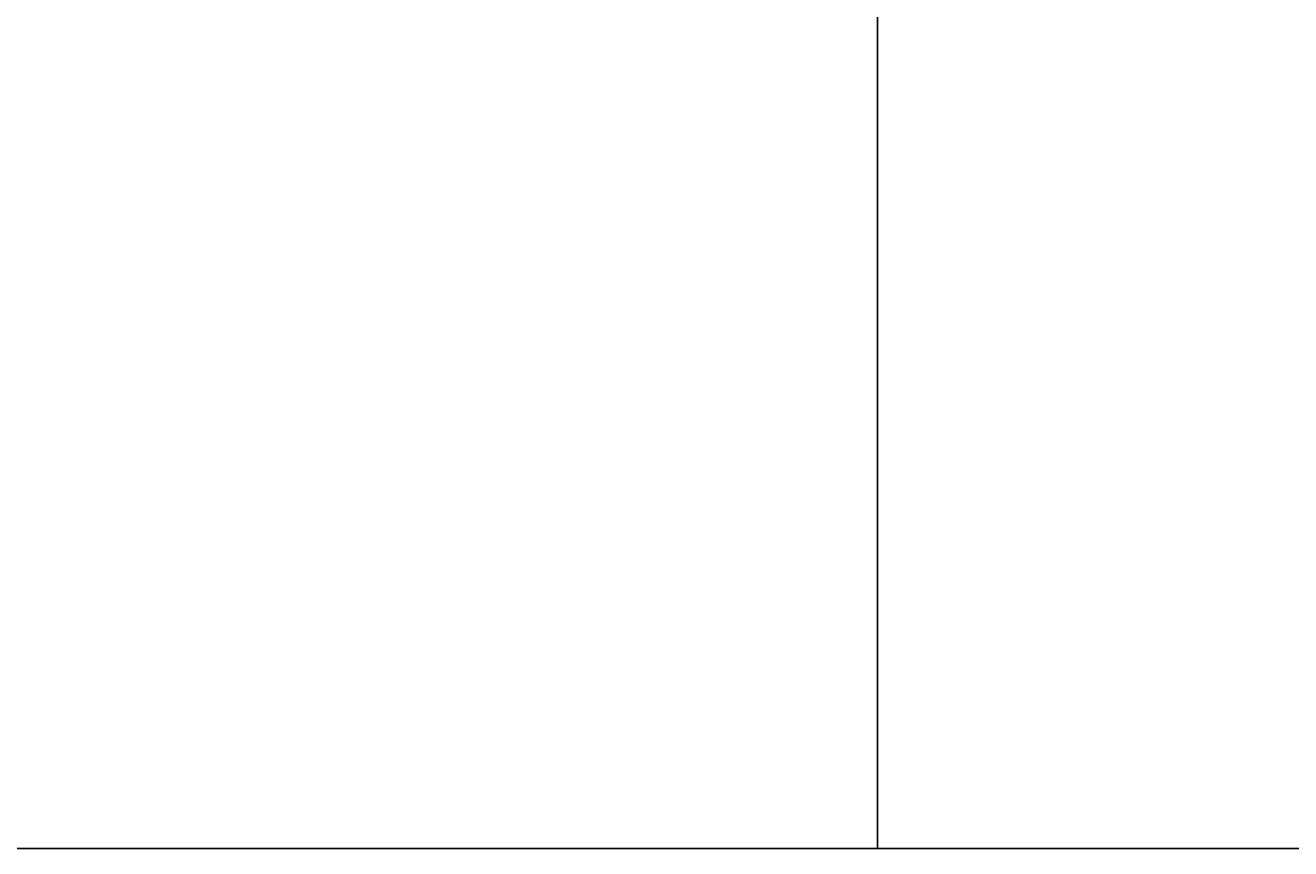
# Model space of a CAD drawing. Units: inches. Extents: x 35362 to 73946, y 43607 to 67532.
# Tile 133 of 134: x 68484 to 70544, y 43607 to 44948. Entities that reach past the tile are written whole.
import ezdxf

# ---------------------------------------------------------------- set-up
doc = ezdxf.new("R2010")
doc.units = ezdxf.units.IN
doc.header["$MEASUREMENT"] = 0
doc.layers.add('A-ANNO-DIMS', color=2, linetype='Continuous', lineweight=18)
doc.styles.get("Standard").update_dxf_attribs({"font": 'arial.ttf'})
doc.dimstyles.get("Standard").update_dxf_attribs({"dimtxt": 0.18, "dimasz": 0.18, "dimexe": 0.18, "dimexo": 0.0625, "dimgap": 0.09, "dimtad": 0, "dimtih": 1, "dimtoh": 1, "dimdec": 4, "dimzin": 0, "dimdsep": 46, "dimtxsty": 'Standard', "dimcen": 0.09, "dimadec": 0, "dimazin": 0, "dimtfac": 1, "dimtdec": 4, "dimtofl": 0, "dimtmove": 0, "dimatfit": 3, "dimfxl": 1, "dimtolj": 1, "dimtzin": 0, "dimarcsym": 0})

# ---------------------------------------------------------------- blocks, each defined once
blk = doc.blocks.new('*D5')
at = {"layer": 'A-ANNO-DIMS', "color": 0, "lineweight": -2, "transparency": 16777216}
for p, q in [((37121.949085, 46919.318283), (37121.949085, 43606.678996)), ((69871.496302, 45449.831951), (69871.496302, 43606.678996)), ((37122.129085, 43606.858996), (53496.2943647142, 43606.858996)), ((69871.316302, 43606.858996), (53497.15102228581, 43606.858996))]:
    blk.add_line(p, q, dxfattribs=at)
at = {"layer": 'A-ANNO-DIMS', "color": 0, "transparency": 16777216}
for points in [[(37122.129085, 43606.888996), (37122.129085, 43606.828996), (37121.949085, 43606.858996)], [(69871.316302, 43606.888996), (69871.316302, 43606.828996), (69871.496302, 43606.858996)]]:
    blk.add_solid(points, dxfattribs=at)
at = {"layer": 'Defpoints', "color": 0, "transparency": 16777216}
for p in [(37121.949085, 46919.380783), (69871.496302, 45449.894451), (69871.496302, 43606.858996)]:
    blk.add_point(p, dxfattribs=at)
at = {"layer": 'A-ANNO-DIMS', "color": 0, "transparency": 16777216, "insert": (53496.7226935, 43606.858996), "char_height": 0.18, "attachment_point": 5}
blk.add_mtext('\\A1;32750', dxfattribs=at)
blk = doc.blocks.new('*D6')
at = {"layer": 'A-ANNO-DIMS', "color": 0, "lineweight": -2, "transparency": 16777216}
for p, q in [((72185.645666, 53702.123839), (72185.645666, 43606.678996)), ((69871.496302, 45449.831951), (69871.496302, 43606.678996)), ((69871.67630199999, 43606.858996), (71028.21104539152, 43606.858996)), ((72185.465666, 43606.858996), (71028.93092260844, 43606.858996))]:
    blk.add_line(p, q, dxfattribs=at)
at = {"layer": 'A-ANNO-DIMS', "color": 0, "transparency": 16777216}
for points in [[(69871.67630199999, 43606.888996), (69871.67630199999, 43606.828996), (69871.496302, 43606.858996)], [(72185.465666, 43606.888996), (72185.465666, 43606.828996), (72185.645666, 43606.858996)]]:
    blk.add_solid(points, dxfattribs=at)
at = {"layer": 'Defpoints', "color": 0, "transparency": 16777216}
for p in [(72185.645666, 53702.186339), (69871.496302, 45449.894451), (72185.645666, 43606.858996)]:
    blk.add_point(p, dxfattribs=at)
at = {"layer": 'A-ANNO-DIMS', "color": 0, "transparency": 16777216, "insert": (71028.57098399999, 43606.858996), "char_height": 0.18, "attachment_point": 5}
blk.add_mtext('\\A1;2314', dxfattribs=at)

msp = doc.modelspace()

# ---------------------------------------------------------------- dimensions: what is measured, and where the dimension line sits
at = {"layer": 'A-ANNO-DIMS'}
for base, p1, p2, picture, middle in [((72185.645666, 43606.858996), (69871.496302, 45449.894451), (72185.645666, 53702.186339), '*D6', (71028.57098399999, 43606.858996)), ((69871.496302, 43606.858996), (37121.949085, 46919.380783), (69871.496302, 45449.894451), '*D5', (53496.7226935, 43606.858996))]:
    dim = msp.add_linear_dim(base=base, p1=p1, p2=p2, dimstyle='Standard', override={"dimdec": 0, "dimlfac": 1, "dimrnd": 0, "dimzin": 0, "dimdsep": 46, "dimlunit": 2}, dxfattribs=at)
    dim.commit()
    dim.dimension.update_dxf_attribs({"geometry": picture, "text_midpoint": middle})

doc.saveas('drawing.dxf')
